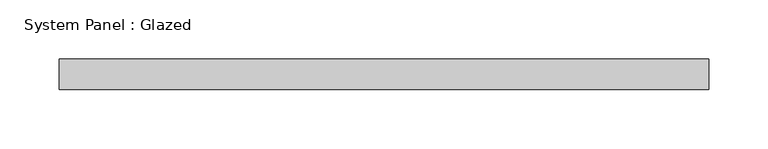
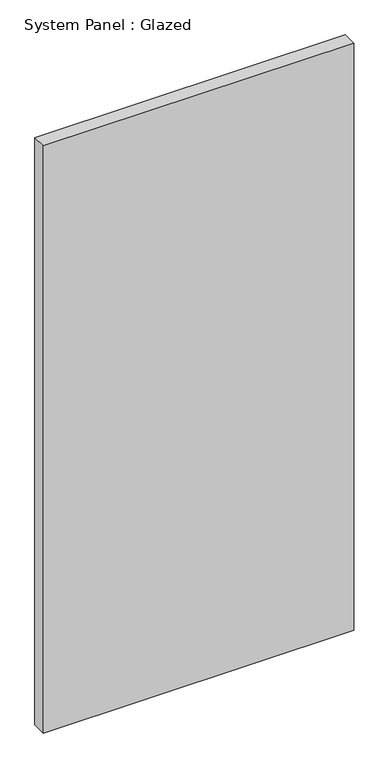
"""IFC4 building model written with IfcOpenShell, lengths in millimetres: plate geometry, System Panel : Glazed."""

from ifc_helpers import new_model, si_unit, origin, origin_with_axes, place, context, project, spatial, polyline, outline, extrude, source, transform, mapped, element, save


def system_panel_glazed_fcede64b(model_context):
    return source(origin(), model_context, "Body", "SweptSolid", [
        extrude(outline(polyline([(273.05, 19.05), (-273.05, 19.05), (-273.05, 44.45), (273.05, 44.45), (273.05, 19.05)])), origin_with_axes(), (0.0, 0.0, 1.0), 1092.2),
    ])


if __name__ == "__main__":
    model = new_model("IFC4")
    model_context = context("Model", 3, world=origin())
    ifc_project = project(units=[si_unit("LENGTHUNIT", "METRE", prefix="MILLI")], contexts=[model_context])
    site = spatial("IfcSite", under=ifc_project)
    building = spatial("IfcBuilding", under=site)
    placement = place(None, origin())
    system_panel_glazed_shape = system_panel_glazed_fcede64b(model_context)
    element("IfcPlate", 1, ObjectType="System Panel : Glazed", at=placement, inside=building, context=model_context, shape_type="MappedRepresentation", body=[
        mapped(system_panel_glazed_shape, transform((0.0, 0.0, 0.0), x_axis=(1.0, 0.0, 0.0), y_axis=(0.0, 1.0, 0.0), z_axis=(0.0, 0.0, 1.0))),
    ])
    save(model, "model.ifc")

# Revit data of these elements
# Type "System Panel : Glazed"
#   Construction Type Id = "GSP4R"
#   Analytic Construction = "1/8 in Pilkington single glazing"
#   Visual Light Transmittance = 0.9
#   Solar Heat Gain Coefficient = 0.86
#   Heat Transfer Coefficient (U) = 1.18115 BTU/(h·ft²·°F)
#   Define Thermal Properties by = 1
# Element 1 (IfcPlate, "System Panel : Glazed")
#   Materials on its faces: "Glass"
# Materials
#   "Glass": class "Glass", colour RGB 0 128 192, transparency 0.75, Description = "Soda Lime Glass", Cost = 0
